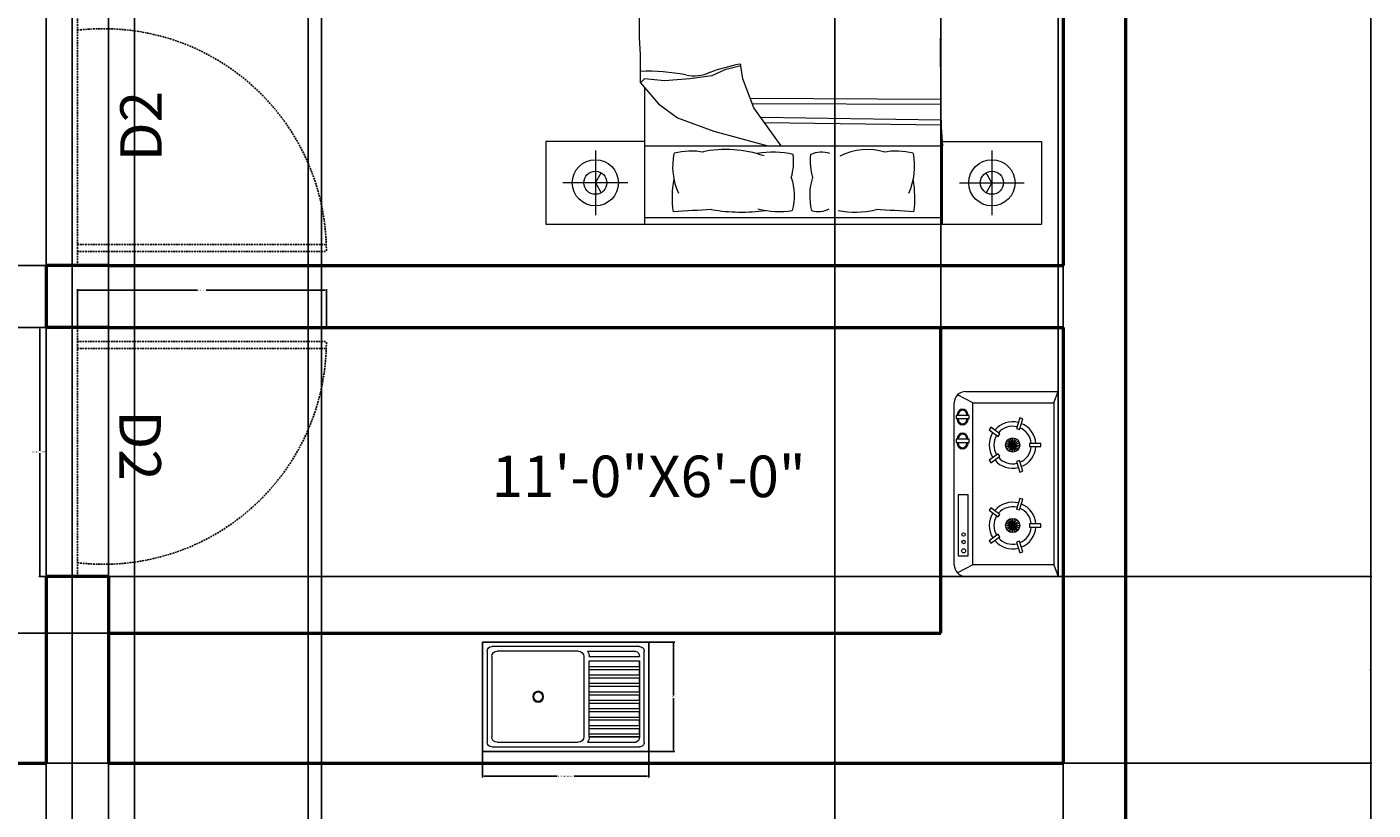
# Model space of a CAD drawing. Units: inches. Extents: x 3 to 576, y -689 to 51.
# Tile 19 of 21: x 381 to 576, y -261 to -148. Entities that reach past the tile are written whole.
import ezdxf

# ---------------------------------------------------------------- set-up
doc = ezdxf.new("R2010")
doc.units = ezdxf.units.IN
doc.header["$MEASUREMENT"] = 0
doc.linetypes.add('DASHED2', pattern=[0.375, 0.25, -0.125])
for name, color, linetype, lineweight in [('A-ANNO-DIMS', 2, 'Continuous', 18), ('A-ANNO-TEXT', 3, 'Continuous', 18), ('A-AREA-IDEN', 7, 'Continuous', 18), ('A-DOOR', 4, 'DASHED2', 25), ('A-EQPM', 8, 'Continuous', 18), ('A-FLOR-FIXT', 9, 'Continuous', 18), ('A-FURN', 8, 'Continuous', 18), ('A-WALL', 7, 'Continuous', 50)]:
    doc.layers.add(name, color=color, linetype=linetype, lineweight=lineweight)
doc.styles.get("Standard").update_dxf_attribs({"font": 'arial.ttf'})
doc.dimstyles.get("Standard").update_dxf_attribs({"dimtxt": 0.18, "dimasz": 0.18, "dimexe": 0.18, "dimexo": 0.0625, "dimgap": 0.09, "dimtad": 0, "dimtih": 1, "dimtoh": 1, "dimdec": 0, "dimzin": 0, "dimdsep": 46, "dimlunit": 3, "dimtxsty": 'Standard', "dimcen": 0.09, "dimadec": 0, "dimazin": 0, "dimtfac": 1, "dimtdec": 0, "dimtofl": 0, "dimtmove": 0, "dimatfit": 3, "dimfxl": 1, "dimtolj": 1, "dimtzin": 0, "dimarcsym": 0})

# ---------------------------------------------------------------- blocks, each defined once
blk = doc.blocks.new('М12 540х820')
for p, q in [((0, 540), (-820, 540)), ((-820, 540), (-820, 0)), ((0, 0), (0, 540)), ((-797.5, 495), (-797.5, 45)), ((-45, 517.5), (-775, 517.5)), ((-775, 468), (-775, 72)), ((-347.5, 495), (-748, 495)), ((-320.5, 468), (-320.5, 72)), ((-301.7, 495), (-64.8, 495)), ((-293.7, 468), (-293.7, 472.5)), ((-293.7, 468), (-45, 468)), ((-45, 469.5), (-45, 468)), ((-22.5, 45), (-22.5, 495)), ((-293.7, 446.6), (-45, 446.6)), ((-293.7, 419.6), (-293.7, 446.6)), ((-293.7, 419.6), (-45, 419.6)), ((-293.7, 405), (-45, 405)), ((-293.7, 378), (-293.7, 405)), ((-45, 419.6), (-45, 446.6)), ((-45, 378), (-45, 405)), ((-293.7, 378), (-45, 378)), ((-293.7, 336.4), (-293.7, 363.4)), ((-293.7, 363.4), (-45, 363.4)), ((-293.7, 336.4), (-45, 336.4)), ((-45, 336.4), (-45, 363.4)), ((-293.7, 294.7), (-293.7, 321.7)), ((-293.7, 321.7), (-45, 321.7)), ((-293.7, 294.7), (-45, 294.7)), ((-293.7, 253.1), (-293.7, 280.1)), ((-293.7, 280.1), (-45, 280.1)), ((-45, 294.7), (-45, 321.7)), ((-45, 253.1), (-45, 280.1)), ((-293.7, 253.1), (-45, 253.1)), ((-293.7, 211.5), (-293.7, 238.5)), ((-293.7, 238.5), (-45, 238.5)), ((-293.7, 211.5), (-45, 211.5)), ((-45, 211.5), (-45, 238.5)), ((-293.7, 169.9), (-293.7, 196.9)), ((-293.7, 196.9), (-45, 196.9)), ((-293.7, 169.9), (-45, 169.9)), ((-293.7, 128.2), (-293.7, 155.2)), ((-293.7, 155.2), (-45, 155.2)), ((-45, 169.9), (-45, 196.9)), ((-45, 128.2), (-45, 155.2)), ((-293.7, 128.2), (-45, 128.2)), ((-293.7, 113.6), (-45, 113.6)), ((-293.7, 86.6), (-293.7, 113.6)), ((-293.7, 86.6), (-45, 86.6)), ((-293.7, 72), (-45, 72)), ((-45, 86.6), (-45, 113.6)), ((-45, 70.5), (-45, 72)), ((-820, 0), (0, 0)), ((-775, 22.5), (-45, 22.5)), ((-748, 45), (-347.5, 45)), ((-301.7, 45), (-64.8, 45))]:
    blk.add_line(p, q)
at = {"ltscale": 0.06}
for p, q in [((-820, 0), (-820, 540)), ((-820, 540), (0, 540)), ((0, 540), (0, 536.9)), ((0, 536.9), (0, 0)), ((-293.7, 446.6), (-45, 446.6)), ((-293.7, 405), (-293.7, 446.6)), ((-293.7, 363.4), (-293.7, 405)), ((-45, 446.6), (-45, 419.6)), ((-45, 419.6), (-45, 378)), ((-293.7, 321.7), (-293.7, 363.4)), ((-45, 378), (-45, 336.4)), ((-45, 336.4), (-45, 294.7)), ((-293.7, 280.1), (-293.7, 321.7)), ((-293.7, 238.5), (-293.7, 280.1)), ((-45, 294.7), (-45, 253.1)), ((-293.7, 196.9), (-293.7, 238.5)), ((-45, 253.1), (-45, 211.5)), ((-45, 211.5), (-45, 169.9)), ((-293.7, 155.2), (-293.7, 196.9)), ((-293.7, 113.6), (-293.7, 155.2)), ((-45, 169.9), (-45, 128.2)), ((-293.7, 72), (-293.7, 113.6)), ((-45, 72), (-293.7, 72)), ((-45, 128.2), (-45, 86.6)), ((-45, 86.6), (-45, 72)), ((0, 0), (-820, 0))]:
    blk.add_line(p, q, dxfattribs=at)
at = {"extrusion": (0, 0, -1)}
for centre, major_axis, start_param, end_param in [((-775, 495), (-15.9, 15.9), -0.785398, 0.785398), ((-775, 495), (-15.9, 15.9), -0.785398, 0.785398), ((-748, 468), (-19.1, -19.1), 0.785398, 2.356194), ((-748, 468), (-19.1, -19.1), 0.785398, 2.356194), ((-347.5, 468), (-19.1, 19.1), 0.785398, 2.356194), ((-347.5, 468), (-19.1, 19.1), 0.785398, 2.356194), ((-343.2, 468), (-35, 35), 1.779263, 2.356194), ((-343.2, 468), (-35, 35), 1.779263, 2.356192), ((-343.2, 468), (-35, 35), 2.356192, 2.356194), ((-72.3, 468.8), (-19.3, 19.3), 1.0328, 2.38382), ((-72.3, 468.8), (-19.3, 19.3), 1.0328, 1.064673), ((-72.3, 468.8), (-19.3, 19.3), 1.064673, 2.328569), ((-45, 495), (-15.9, -15.9), 2.356194, 3.926991), ((-45, 495), (-15.9, -15.9), 2.356194, 3.926991), ((-72.3, 468.8), (-19.3, 19.3), 2.328569, 2.38382), ((-545.5, 270), (-19.1, -19.1), 3.926991, 10.210176), ((-545.5, 270), (-19.1, -19.1), 3.926991, 10.210176), ((-545.5, 270), (-15.9, -15.9), 3.926991, 10.210176), ((-545.5, 270), (-15.9, -15.9), 3.926991, 10.210176), ((-748, 72), (-19.1, 19.1), 3.926991, 5.497787), ((-748, 72), (-19.1, 19.1), 3.926991, 5.497787), ((-347.5, 72), (-19.1, -19.1), 3.926991, 5.497787), ((-347.5, 72), (-19.1, -19.1), 3.926991, 5.497787), ((-343.2, 72), (-35, -35), 3.926991, 4.503922), ((-343.2, 72), (-35, -35), 3.926991, 4.503922), ((-72.3, 71.2), (-19.3, -19.3), 3.899365, 5.250385), ((-72.3, 71.2), (-19.3, -19.3), 3.954617, 5.218512), ((-72.3, 71.2), (-19.3, -19.3), 3.899365, 3.954617), ((-775, 45), (-15.9, -15.9), 5.497787, 7.068583), ((-775, 45), (-15.9, -15.9), 5.497787, 7.068583), ((-72.3, 71.2), (-19.3, -19.3), 5.218512, 5.250385), ((-45, 45), (-15.9, 15.9), 2.356194, 3.926991), ((-45, 45), (-15.9, 15.9), 2.356194, 3.926991)]:
    blk.add_ellipse(centre, major_axis=major_axis, ratio=1, start_param=start_param, end_param=end_param, dxfattribs=at)
blk = doc.blocks.new('DOOR-SWING-900')
for p, q in [((35.95, 36), (35.95, 34)), ((36, 2), (35.95, 34)), ((36, 2), (0, 2)), ((36, 0), (36, 2))]:
    blk.add_line(p, q)
blk.add_arc((32.22, 2), 32.22, 83.347, 180)
blk = doc.blocks.new('*D15')
at = {"layer": 'A-ANNO-DIMS', "color": 0, "lineweight": -2, "transparency": 16777216}
for p, q in [((388.72, -191.31), (383.2, -191.31)), ((383.38, -191.49), (383.37, -209.12)), ((383.37, -227.13), (383.37, -209.49)), ((388.71, -227.31), (383.19, -227.31))]:
    blk.add_line(p, q, dxfattribs=at)
at = {"layer": 'A-ANNO-DIMS', "color": 0, "transparency": 16777216}
for points in [[(383.35, -191.49), (383.41, -191.49), (383.38, -191.31)], [(383.34, -227.13), (383.4, -227.13), (383.37, -227.31)]]:
    blk.add_solid(points, dxfattribs=at)
at = {"layer": 'Defpoints', "color": 0, "transparency": 16777216}
for p in [(388.78, -191.31), (383.37, -227.31), (388.77, -227.31)]:
    blk.add_point(p, dxfattribs=at)
at = {"layer": 'A-ANNO-DIMS', "color": 0, "transparency": 16777216, "insert": (383.37, -209.31), "char_height": 0.18, "attachment_point": 5}
blk.add_mtext('\\A1;DOOR D2 3\'-0" TYP.', dxfattribs=at)
blk = doc.blocks.new('*D16')
at = {"layer": 'A-ANNO-DIMS', "color": 0, "lineweight": -2, "transparency": 16777216}
for p, q in [((388.78, -191.25), (388.78, -185.73)), ((388.96, -185.91), (406.14, -185.91)), ((424.6, -185.92), (407.42, -185.91)), ((424.78, -191.25), (424.78, -185.74))]:
    blk.add_line(p, q, dxfattribs=at)
at = {"layer": 'A-ANNO-DIMS', "color": 0, "transparency": 16777216}
for points in [[(388.96, -185.88), (388.96, -185.94), (388.78, -185.91)], [(424.6, -185.89), (424.6, -185.95), (424.78, -185.92)]]:
    blk.add_solid(points, dxfattribs=at)
at = {"layer": 'Defpoints', "color": 0, "transparency": 16777216}
for p in [(388.78, -185.91), (388.78, -191.31), (424.78, -191.32)]:
    blk.add_point(p, dxfattribs=at)
at = {"layer": 'A-ANNO-DIMS', "color": 0, "transparency": 16777216, "insert": (406.78, -185.91), "char_height": 0.18, "attachment_point": 5}
blk.add_mtext('\\A1;3\'-0" TYP.', dxfattribs=at)
blk = doc.blocks.new('*D25')
at = {"layer": 'A-ANNO-DIMS', "color": 0, "lineweight": -2, "transparency": 16777216}
for p, q in [((447.36, -252.65), (447.36, -256.37)), ((471.37, -252.65), (471.37, -256.37)), ((447.54, -256.19), (458.13, -256.19)), ((471.19, -256.19), (460.61, -256.19))]:
    blk.add_line(p, q, dxfattribs=at)
at = {"layer": 'A-ANNO-DIMS', "color": 0, "transparency": 16777216}
for points in [[(447.54, -256.16), (447.54, -256.22), (447.36, -256.19)], [(471.19, -256.16), (471.19, -256.22), (471.37, -256.19)]]:
    blk.add_solid(points, dxfattribs=at)
at = {"layer": 'Defpoints', "color": 0, "transparency": 16777216}
for p in [(447.36, -252.59), (471.37, -252.59), (471.37, -256.19)]:
    blk.add_point(p, dxfattribs=at)
at = {"layer": 'A-ANNO-DIMS', "color": 0, "transparency": 16777216, "insert": (459.37, -256.19), "char_height": 0.18, "attachment_point": 5}
blk.add_mtext('\\A1;KITCHEN SINK 2\'-0"', dxfattribs=at)
blk = doc.blocks.new('*D26')
at = {"layer": 'A-ANNO-DIMS', "color": 0, "lineweight": -2, "transparency": 16777216}
for p, q in [((471.43, -236.78), (475.15, -236.78)), ((474.97, -236.96), (474.97, -244.5)), ((474.97, -252.41), (474.97, -244.87)), ((471.43, -252.59), (475.15, -252.59))]:
    blk.add_line(p, q, dxfattribs=at)
at = {"layer": 'A-ANNO-DIMS', "color": 0, "transparency": 16777216}
for points in [[(474.94, -236.96), (475, -236.96), (474.97, -236.78)], [(474.94, -252.41), (475, -252.41), (474.97, -252.59)]]:
    blk.add_solid(points, dxfattribs=at)
at = {"layer": 'Defpoints', "color": 0, "transparency": 16777216}
for p in [(471.37, -236.78), (474.97, -236.78), (471.37, -252.59)]:
    blk.add_point(p, dxfattribs=at)
at = {"layer": 'A-ANNO-DIMS', "color": 0, "transparency": 16777216, "insert": (474.97, -244.68), "char_height": 0.18, "attachment_point": 5}
blk.add_mtext('\\A1;1\'-4"', dxfattribs=at)
blk = doc.blocks.new('*D39')
at = {"layer": 'A-ANNO-DIMS', "color": 0, "lineweight": -2, "transparency": 16777216}
for p, q in [((540.36, 15.69), (575.92, 15.69)), ((575.74, 15.51), (575.74, -318.63)), ((575.74, -653.13), (575.74, -318.99)), ((540.36, -653.31), (575.92, -653.31))]:
    blk.add_line(p, q, dxfattribs=at)
at = {"layer": 'A-ANNO-DIMS', "color": 0, "transparency": 16777216}
for points in [[(575.71, 15.51), (575.77, 15.51), (575.74, 15.69)], [(575.71, -653.13), (575.77, -653.13), (575.74, -653.31)]]:
    blk.add_solid(points, dxfattribs=at)
at = {"layer": 'Defpoints', "color": 0, "transparency": 16777216}
for p in [(540.29, 15.69), (540.29, -653.31), (575.74, -653.31)]:
    blk.add_point(p, dxfattribs=at)
at = {"layer": 'A-ANNO-DIMS', "color": 0, "transparency": 16777216, "insert": (575.74, -318.81), "char_height": 0.18, "attachment_point": 5}
blk.add_mtext('\\A1;55\'-9"', dxfattribs=at)
blk = doc.blocks.new('*D65')
at = {"layer": 'A-ANNO-DIMS', "color": 0, "lineweight": -2, "transparency": 16777216}
for p, q in [((531.23, -50.31), (2.66, -50.31)), ((2.84, -50.49), (2.84, -116.13)), ((2.84, -182.13), (2.84, -116.49)), ((531.23, -182.31), (2.66, -182.31))]:
    blk.add_line(p, q, dxfattribs=at)
at = {"layer": 'A-ANNO-DIMS', "color": 0, "transparency": 16777216}
for points in [[(2.81, -50.49), (2.87, -50.49), (2.84, -50.31)], [(2.81, -182.13), (2.87, -182.13), (2.84, -182.31)]]:
    blk.add_solid(points, dxfattribs=at)
at = {"layer": 'Defpoints', "color": 0, "transparency": 16777216}
for p in [(531.29, -50.31), (2.84, -182.31), (531.29, -182.31)]:
    blk.add_point(p, dxfattribs=at)
at = {"layer": 'A-ANNO-DIMS', "color": 0, "transparency": 16777216, "insert": (2.84, -116.31), "char_height": 0.18, "attachment_point": 5}
blk.add_mtext('\\A1;11\'-0"', dxfattribs=at)
blk = doc.blocks.new('*D66')
at = {"layer": 'A-ANNO-DIMS', "color": 0, "lineweight": -2, "transparency": 16777216}
for p, q in [((531.23, -182.31), (2.66, -182.31)), ((2.84, -182.49), (2.84, -186.63)), ((2.84, -191.13), (2.84, -186.99)), ((531.23, -191.31), (2.66, -191.31))]:
    blk.add_line(p, q, dxfattribs=at)
at = {"layer": 'A-ANNO-DIMS', "color": 0, "transparency": 16777216}
for points in [[(2.81, -182.49), (2.87, -182.49), (2.84, -182.31)], [(2.81, -191.13), (2.87, -191.13), (2.84, -191.31)]]:
    blk.add_solid(points, dxfattribs=at)
at = {"layer": 'Defpoints', "color": 0, "transparency": 16777216}
for p in [(531.29, -182.31), (2.84, -191.31), (531.29, -191.31)]:
    blk.add_point(p, dxfattribs=at)
at = {"layer": 'A-ANNO-DIMS', "color": 0, "transparency": 16777216, "insert": (2.84, -186.81), "char_height": 0.18, "attachment_point": 5}
blk.add_mtext('\\A1;0\'-9"', dxfattribs=at)
blk = doc.blocks.new('*D67')
at = {"layer": 'A-ANNO-DIMS', "color": 0, "lineweight": -2, "transparency": 16777216}
for p, q in [((531.23, -191.31), (2.66, -191.31)), ((2.84, -191.49), (2.84, -222.63)), ((2.84, -254.13), (2.84, -222.99)), ((531.23, -254.31), (2.66, -254.31))]:
    blk.add_line(p, q, dxfattribs=at)
at = {"layer": 'A-ANNO-DIMS', "color": 0, "transparency": 16777216}
for points in [[(2.81, -191.49), (2.87, -191.49), (2.84, -191.31)], [(2.81, -254.13), (2.87, -254.13), (2.84, -254.31)]]:
    blk.add_solid(points, dxfattribs=at)
at = {"layer": 'Defpoints', "color": 0, "transparency": 16777216}
for p in [(531.29, -191.31), (2.84, -254.31), (531.29, -254.31)]:
    blk.add_point(p, dxfattribs=at)
at = {"layer": 'A-ANNO-DIMS', "color": 0, "transparency": 16777216, "insert": (2.84, -222.81), "char_height": 0.18, "attachment_point": 5}
blk.add_mtext('\\A1;5\'-3"', dxfattribs=at)
blk = doc.blocks.new('*D68')
at = {"layer": 'A-ANNO-DIMS', "color": 0, "lineweight": -2, "transparency": 16777216}
for p, q in [((531.23, -254.31), (2.66, -254.31)), ((2.84, -254.49), (2.84, -258.63)), ((2.84, -263.13), (2.84, -258.99)), ((531.23, -263.31), (2.66, -263.31))]:
    blk.add_line(p, q, dxfattribs=at)
at = {"layer": 'A-ANNO-DIMS', "color": 0, "transparency": 16777216}
for points in [[(2.81, -254.49), (2.87, -254.49), (2.84, -254.31)], [(2.81, -263.13), (2.87, -263.13), (2.84, -263.31)]]:
    blk.add_solid(points, dxfattribs=at)
at = {"layer": 'Defpoints', "color": 0, "transparency": 16777216}
for p in [(531.29, -254.31), (2.84, -263.31), (531.29, -263.31)]:
    blk.add_point(p, dxfattribs=at)
at = {"layer": 'A-ANNO-DIMS', "color": 0, "transparency": 16777216, "insert": (2.84, -258.81), "char_height": 0.18, "attachment_point": 5}
blk.add_mtext('\\A1;0\'-9"', dxfattribs=at)
blk = doc.blocks.new('*D94')
at = {"layer": 'A-ANNO-DIMS', "color": 0, "lineweight": -2, "transparency": 16777216}
for p, q in [((393.29, -136.9), (393.29, -688.94)), ((422.14, -136.9), (422.14, -688.94)), ((393.47, -688.76), (407.39, -688.76)), ((421.96, -688.76), (408.05, -688.76))]:
    blk.add_line(p, q, dxfattribs=at)
at = {"layer": 'A-ANNO-DIMS', "color": 0, "transparency": 16777216}
for points in [[(393.47, -688.73), (393.47, -688.79), (393.29, -688.76)], [(421.96, -688.73), (421.96, -688.79), (422.14, -688.76)]]:
    blk.add_solid(points, dxfattribs=at)
at = {"layer": 'Defpoints', "color": 0, "transparency": 16777216}
for p in [(393.29, -136.84), (422.14, -136.84), (422.14, -688.76)]:
    blk.add_point(p, dxfattribs=at)
at = {"layer": 'A-ANNO-DIMS', "color": 0, "transparency": 16777216, "insert": (407.72, -688.76), "char_height": 0.18, "attachment_point": 5}
blk.add_mtext('\\A1;2\'-5"', dxfattribs=at)
blk = doc.blocks.new('*D96')
at = {"layer": 'A-ANNO-DIMS', "color": 0, "lineweight": -2, "transparency": 16777216}
for p, q in [((397.02, -506.04), (397.02, 51.32)), ((397.2, 51.14), (410.22, 51.14)), ((423.91, 51.14), (410.89, 51.14)), ((424.09, -506.04), (424.09, 51.32))]:
    blk.add_line(p, q, dxfattribs=at)
at = {"layer": 'A-ANNO-DIMS', "color": 0, "transparency": 16777216}
for points in [[(397.2, 51.17), (397.2, 51.11), (397.02, 51.14)], [(423.91, 51.17), (423.91, 51.11), (424.09, 51.14)]]:
    blk.add_solid(points, dxfattribs=at)
at = {"layer": 'Defpoints', "color": 0, "transparency": 16777216}
for p in [(424.09, 51.14), (397.02, -506.1), (424.09, -506.1)]:
    blk.add_point(p, dxfattribs=at)
at = {"layer": 'A-ANNO-DIMS', "color": 0, "transparency": 16777216, "insert": (410.56, 51.14), "char_height": 0.18, "attachment_point": 5}
blk.add_mtext('\\A1;2\'-3"', dxfattribs=at)
blk = doc.blocks.new('*D103')
at = {"layer": 'A-ANNO-DIMS', "color": 0, "lineweight": -2, "transparency": 16777216}
for p, q in [((498.29, -50.37), (498.29, -688.94)), ((531.29, -50.37), (531.29, -688.94)), ((498.47, -688.76), (514.46, -688.76)), ((531.11, -688.76), (515.12, -688.76))]:
    blk.add_line(p, q, dxfattribs=at)
at = {"layer": 'A-ANNO-DIMS', "color": 0, "transparency": 16777216}
for points in [[(498.47, -688.73), (498.47, -688.79), (498.29, -688.76)], [(531.11, -688.73), (531.11, -688.79), (531.29, -688.76)]]:
    blk.add_solid(points, dxfattribs=at)
at = {"layer": 'Defpoints', "color": 0, "transparency": 16777216}
for p in [(498.29, -50.31), (531.29, -50.31), (531.29, -688.76)]:
    blk.add_point(p, dxfattribs=at)
at = {"layer": 'A-ANNO-DIMS', "color": 0, "transparency": 16777216, "insert": (514.79, -688.76), "char_height": 0.18, "attachment_point": 5}
blk.add_mtext('\\A1;2\'-9"', dxfattribs=at)
blk = doc.blocks.new('*D105')
at = {"layer": 'A-ANNO-DIMS', "color": 0, "lineweight": -2, "transparency": 16777216}
for p, q in [((393.36, -227.31), (575.92, -227.31)), ((575.74, -227.49), (575.74, -240.63)), ((575.74, -254.13), (575.74, -240.99)), ((393.36, -254.31), (575.92, -254.31))]:
    blk.add_line(p, q, dxfattribs=at)
at = {"layer": 'A-ANNO-DIMS', "color": 0, "transparency": 16777216}
for points in [[(575.71, -227.49), (575.77, -227.49), (575.74, -227.31)], [(575.71, -254.13), (575.77, -254.13), (575.74, -254.31)]]:
    blk.add_solid(points, dxfattribs=at)
at = {"layer": 'Defpoints', "color": 0, "transparency": 16777216}
for p in [(393.29, -227.31), (393.29, -254.31), (575.74, -254.31)]:
    blk.add_point(p, dxfattribs=at)
at = {"layer": 'A-ANNO-DIMS', "color": 0, "transparency": 16777216, "insert": (575.74, -240.81), "char_height": 0.18, "attachment_point": 5}
blk.add_mtext('\\A1;2\'-3"', dxfattribs=at)
blk = doc.blocks.new('*D116')
at = {"layer": 'A-ANNO-DIMS', "color": 0, "lineweight": -2, "transparency": 16777216}
for p, q in [((360.29, -134.37), (360.29, -688.94)), ((384.29, -134.37), (384.29, -688.94)), ((360.47, -688.76), (371.96, -688.76)), ((384.11, -688.76), (372.62, -688.76))]:
    blk.add_line(p, q, dxfattribs=at)
at = {"layer": 'A-ANNO-DIMS', "color": 0, "transparency": 16777216}
for points in [[(360.47, -688.73), (360.47, -688.79), (360.29, -688.76)], [(384.11, -688.73), (384.11, -688.79), (384.29, -688.76)]]:
    blk.add_solid(points, dxfattribs=at)
at = {"layer": 'Defpoints', "color": 0, "transparency": 16777216}
for p in [(360.29, -134.31), (384.29, -134.31), (384.29, -688.76)]:
    blk.add_point(p, dxfattribs=at)
at = {"layer": 'A-ANNO-DIMS', "color": 0, "transparency": 16777216, "insert": (372.29, -688.76), "char_height": 0.18, "attachment_point": 5}
blk.add_mtext('\\A1;2\'-0"', dxfattribs=at)
blk = doc.blocks.new('*D118')
at = {"layer": 'A-ANNO-DIMS', "color": 0, "lineweight": -2, "transparency": 16777216}
for p, q in [((352.02, -506.25), (352.02, 51.32)), ((352.2, 51.14), (369.69, 51.14)), ((387.84, 51.14), (370.35, 51.14)), ((388.02, -506.25), (388.02, 51.32))]:
    blk.add_line(p, q, dxfattribs=at)
at = {"layer": 'A-ANNO-DIMS', "color": 0, "transparency": 16777216}
for points in [[(352.2, 51.17), (352.2, 51.11), (352.02, 51.14)], [(387.84, 51.17), (387.84, 51.11), (388.02, 51.14)]]:
    blk.add_solid(points, dxfattribs=at)
at = {"layer": 'Defpoints', "color": 0, "transparency": 16777216}
for p in [(388.02, 51.14), (352.02, -506.31), (388.02, -506.31)]:
    blk.add_point(p, dxfattribs=at)
at = {"layer": 'A-ANNO-DIMS', "color": 0, "transparency": 16777216, "insert": (370.02, 51.14), "char_height": 0.18, "attachment_point": 5}
blk.add_mtext('\\A1;3\'-0"', dxfattribs=at)
blk = doc.blocks.new('*D123')
at = {"layer": 'A-ANNO-DIMS', "color": 0, "lineweight": -2, "transparency": 16777216}
for p, q in [((513.55, -235.5), (2.66, -235.5)), ((2.84, -235.68), (2.84, -244.72)), ((2.84, -254.13), (2.84, -245.08)), ((531.23, -254.31), (2.66, -254.31))]:
    blk.add_line(p, q, dxfattribs=at)
at = {"layer": 'A-ANNO-DIMS', "color": 0, "transparency": 16777216}
for points in [[(2.81, -235.68), (2.87, -235.68), (2.84, -235.5)], [(2.81, -254.13), (2.87, -254.13), (2.84, -254.31)]]:
    blk.add_solid(points, dxfattribs=at)
at = {"layer": 'Defpoints', "color": 0, "transparency": 16777216}
for p in [(513.61, -235.5), (2.84, -254.31), (531.29, -254.31)]:
    blk.add_point(p, dxfattribs=at)
at = {"layer": 'A-ANNO-DIMS', "color": 0, "transparency": 16777216, "insert": (2.84, -244.9), "char_height": 0.18, "attachment_point": 5}
blk.add_mtext('\\A1;1\'-7"', dxfattribs=at)
blk = doc.blocks.new('*D124')
at = {"layer": 'A-ANNO-DIMS', "color": 0, "lineweight": -2, "transparency": 16777216}
for p, q in [((513.61, -235.44), (513.61, 51.32)), ((513.79, 51.14), (521.77, 51.14)), ((530.39, 51.14), (522.41, 51.14)), ((530.57, -227.22), (530.57, 51.32))]:
    blk.add_line(p, q, dxfattribs=at)
at = {"layer": 'A-ANNO-DIMS', "color": 0, "transparency": 16777216}
for points in [[(513.79, 51.17), (513.79, 51.11), (513.61, 51.14)], [(530.39, 51.17), (530.39, 51.11), (530.57, 51.14)]]:
    blk.add_solid(points, dxfattribs=at)
at = {"layer": 'Defpoints', "color": 0, "transparency": 16777216}
for p in [(530.57, 51.14), (530.57, -227.28), (513.61, -235.5)]:
    blk.add_point(p, dxfattribs=at)
at = {"layer": 'A-ANNO-DIMS', "color": 0, "transparency": 16777216, "insert": (522.09, 51.14), "char_height": 0.18, "attachment_point": 5}
blk.add_mtext('\\A1;1\'-5"', dxfattribs=at)

msp = doc.modelspace()

# ---------------------------------------------------------------- linework, layer by layer
at = {"layer": 'A-DOOR'}
for p, q in [((388.79, -179.31), (424.79, -179.31)), ((388.79, -194.31), (424.79, -194.31))]:
    msp.add_line(p, q, dxfattribs=at)
at = {"layer": 'A-EQPM'}
for p, q in [((515.53, -225.61), (515.53, -202.21)), ((518.23, -202.21), (516.01, -201.03)), ((517.2, -200.54), (530.57, -200.54)), ((518.23, -202.21), (529.93, -202.21)), ((518.23, -225.61), (518.23, -202.21)), ((529.93, -202.21), (530.57, -200.54)), ((529.93, -202.21), (529.93, -225.61)), ((530.57, -200.54), (530.57, -227.28)), ((517.68, -204), (515.83, -204)), ((515.83, -204), (515.83, -204.43)), ((517.68, -204.43), (517.68, -204)), ((515.83, -204.43), (517.68, -204.43)), ((520.83, -205.72), (520.57, -206.09)), ((520.57, -206.09), (521.88, -207.04)), ((522.15, -206.67), (520.83, -205.72)), ((525.02, -204.36), (524.52, -205.9)), ((524.52, -205.9), (524.95, -206.04)), ((524.95, -206.04), (525.46, -204.5)), ((525.46, -204.5), (525.02, -204.36)), ((517.68, -207.46), (515.83, -207.46)), ((515.83, -207.46), (515.83, -207.9)), ((515.83, -207.9), (517.68, -207.9)), ((517.68, -207.9), (517.68, -207.46)), ((521.88, -207.04), (522.15, -206.67)), ((523.98, -208.29), (523.01, -207.97)), ((523.98, -208.29), (523.15, -207.68)), ((523.98, -208.29), (523.38, -207.46)), ((523.98, -208.29), (523.67, -207.31)), ((523.98, -208.29), (523.98, -207.26)), ((523.98, -208.29), (524.3, -207.31)), ((523.98, -208.29), (524.59, -207.46)), ((523.98, -208.29), (524.82, -207.68)), ((523.98, -208.29), (524.96, -207.97)), ((526.42, -208.06), (526.42, -208.52)), ((528.04, -208.06), (526.42, -208.06)), ((528.04, -208.52), (528.04, -208.06)), ((521.88, -209.54), (520.57, -210.49)), ((520.83, -210.86), (522.15, -209.91)), ((522.15, -209.91), (521.88, -209.54)), ((523.98, -208.29), (522.96, -208.29)), ((523.98, -208.29), (523.01, -208.61)), ((523.98, -208.29), (523.15, -208.89)), ((523.98, -208.29), (523.38, -209.12)), ((523.98, -208.29), (523.67, -209.27)), ((523.98, -208.29), (523.98, -209.32)), ((523.98, -208.29), (524.3, -209.27)), ((523.98, -208.29), (524.59, -209.12)), ((523.98, -208.29), (524.82, -208.89)), ((523.98, -208.29), (524.96, -208.61)), ((523.98, -208.29), (525.01, -208.29)), ((526.42, -208.52), (528.04, -208.52)), ((520.57, -210.49), (520.83, -210.86)), ((524.95, -210.54), (524.52, -210.68)), ((524.52, -210.68), (525.02, -212.22)), ((525.46, -212.08), (524.95, -210.54)), ((525.02, -212.22), (525.46, -212.08)), ((516.1, -215.48), (516.1, -224.33)), ((517.53, -215.48), (516.1, -215.48)), ((517.53, -224.33), (517.53, -215.48)), ((520.83, -217.36), (520.57, -217.73)), ((520.57, -217.73), (521.88, -218.68)), ((522.15, -218.31), (520.83, -217.36)), ((525.02, -216), (524.52, -217.54)), ((524.52, -217.54), (524.95, -217.68)), ((524.95, -217.68), (525.46, -216.14)), ((525.46, -216.14), (525.02, -216)), ((521.88, -218.68), (522.15, -218.31)), ((523.98, -219.93), (523.01, -219.61)), ((523.98, -219.93), (523.15, -219.33)), ((523.98, -219.93), (523.38, -219.1)), ((523.98, -219.93), (523.67, -218.95)), ((523.98, -219.93), (523.98, -218.9)), ((523.98, -219.93), (524.3, -218.95)), ((523.98, -219.93), (524.59, -219.1)), ((523.98, -219.93), (524.82, -219.33)), ((523.98, -219.93), (524.96, -219.61)), ((526.42, -219.7), (526.42, -220.16)), ((528.04, -219.7), (526.42, -219.7)), ((528.04, -220.16), (528.04, -219.7)), ((521.88, -221.18), (520.57, -222.13)), ((520.83, -222.5), (522.15, -221.55)), ((522.15, -221.55), (521.88, -221.18)), ((523.98, -219.93), (522.96, -219.93)), ((523.98, -219.93), (523.01, -220.25)), ((523.98, -219.93), (523.15, -220.54)), ((523.98, -219.93), (523.38, -220.76)), ((523.98, -219.93), (523.67, -220.91)), ((523.98, -219.93), (525.01, -219.93)), ((523.98, -219.93), (524.96, -220.25)), ((523.98, -219.93), (524.82, -220.54)), ((523.98, -219.93), (524.59, -220.76)), ((523.98, -219.93), (524.3, -220.91)), ((523.98, -219.93), (523.98, -220.96)), ((526.42, -220.16), (528.04, -220.16)), ((520.57, -222.13), (520.83, -222.5)), ((524.95, -222.18), (524.52, -222.32)), ((524.52, -222.32), (525.02, -223.86)), ((525.46, -223.72), (524.95, -222.18)), ((525.02, -223.86), (525.46, -223.72)), ((518.23, -225.61), (516.01, -226.79)), ((516.1, -224.33), (517.53, -224.33)), ((529.93, -225.61), (518.23, -225.61)), ((529.93, -225.61), (530.57, -227.28)), ((530.57, -227.28), (517.2, -227.28))]:
    msp.add_line(p, q, dxfattribs=at)
for centre, radius in [((523.98, -208.29), 1.03), ((523.98, -219.93), 1.03), ((516.89, -221.22), 0.247), ((516.89, -223.59), 0.296), ((516.89, -222.31), 0.247)]:
    msp.add_circle(centre, radius, dxfattribs=at)
for centre, radius, start, end in [((517.2, -202.21), 1.67, 90, 180), ((523.98, -208.29), 3.37, 75.8765, 140.1235), ((523.98, -208.29), 2.71, 76.8365, 139.1635), ((523.98, -208.29), 2.71, 4.8365, 67.1635), ((523.98, -208.29), 3.37, 3.8765, 68.1235), ((523.98, -208.29), 3.37, 147.8765, 212.1235), ((523.98, -208.29), 2.71, 148.8365, 211.1635), ((523.98, -208.29), 2.71, 220.8365, 283.1635), ((523.98, -208.29), 2.71, 292.8365, 355.1635), ((523.98, -208.29), 3.37, 291.8765, 356.1235), ((523.98, -208.29), 3.37, 219.8765, 284.1235), ((523.98, -219.93), 3.37, 75.8765, 140.1235), ((523.98, -219.93), 2.71, 76.8365, 139.1635), ((523.98, -219.93), 2.71, 4.8365, 67.1635), ((523.98, -219.93), 3.37, 3.8765, 68.1235), ((523.98, -219.93), 3.37, 147.8765, 212.1235), ((523.98, -219.93), 2.71, 148.8365, 211.1635), ((523.98, -219.93), 2.71, 220.8365, 283.1635), ((523.98, -219.93), 2.71, 292.8365, 355.1635), ((523.98, -219.93), 3.37, 291.8765, 356.1235), ((523.98, -219.93), 3.37, 219.8765, 284.1235), ((517.2, -225.61), 1.67, 180, 270)]:
    msp.add_arc(centre, radius, start, end, dxfattribs=at)
at = {"layer": 'A-EQPM', "extrusion": (0, 0, -1)}
for centre, major_axis, start_param, end_param in [((516.74, -204.24), (0, -1.2), 1.774361, 4.508825), ((516.74, -204.24), (0, 1.2), 1.73081, 4.552375), ((516.74, -207.71), (0, 1.2), 1.73081, 4.552375), ((516.74, -207.71), (0, -1.2), 1.774361, 4.508825)]:
    msp.add_ellipse(centre, major_axis=major_axis, ratio=0.671641, start_param=start_param, end_param=end_param, dxfattribs=at)
at = {"layer": 'A-EQPM'}
for points, knots in [([(516.12, -204), (516.13, -203.94), (516.15, -203.89), (516.18, -203.76), (516.21, -203.69), (516.26, -203.57), (516.3, -203.51), (516.37, -203.41), (516.41, -203.37), (516.49, -203.3), (516.53, -203.27), (516.61, -203.23), (516.65, -203.22), (516.73, -203.21), (516.77, -203.21), (516.85, -203.23), (516.9, -203.24), (516.98, -203.29), (517.02, -203.32), (517.1, -203.39), (517.14, -203.44), (517.21, -203.54), (517.24, -203.6), (517.29, -203.73), (517.32, -203.8), (517.35, -203.91), (517.35, -203.96), (517.36, -204)], [8.079302, 8.079302, 8.079302, 8.079302, 8.245651, 8.245651, 8.463703, 8.463703, 8.681755, 8.681755, 8.899807, 8.899807, 9.117859, 9.117859, 9.33591, 9.33591, 9.553962, 9.553962, 9.772014, 9.772014, 9.990066, 9.990066, 10.208118, 10.208118, 10.426169, 10.426169, 10.644221, 10.644221, 10.770253, 10.770253, 10.770253, 10.770253]), ([(517.37, -204.43), (517.36, -204.48), (517.35, -204.52), (517.33, -204.64), (517.31, -204.71), (517.26, -204.84), (517.23, -204.91), (517.16, -205.02), (517.12, -205.06), (517.05, -205.15), (517, -205.18), (516.92, -205.23), (516.88, -205.25), (516.81, -205.27), (516.78, -205.27), (516.74, -205.27), (516.7, -205.27), (516.66, -205.27), (516.58, -205.24), (516.54, -205.22), (516.46, -205.16), (516.42, -205.13), (516.34, -205.04), (516.3, -204.99), (516.24, -204.87), (516.21, -204.81), (516.16, -204.67), (516.14, -204.6), (516.13, -204.49), (516.12, -204.46), (516.12, -204.43)], [4.889299, 4.889299, 4.889299, 4.889299, 5.015191, 5.015191, 5.233243, 5.233243, 5.451295, 5.451295, 5.669347, 5.669347, 5.887399, 5.887399, 6.10545, 6.10545, 6.283185, 6.283185, 6.283185, 6.501237, 6.501237, 6.719289, 6.719289, 6.937341, 6.937341, 7.155392, 7.155392, 7.373444, 7.373444, 7.591496, 7.591496, 7.677072, 7.677072, 7.677072, 7.677072]), ([(516.12, -207.46), (516.13, -207.41), (516.15, -207.35), (516.18, -207.22), (516.21, -207.15), (516.26, -207.03), (516.3, -206.97), (516.37, -206.87), (516.41, -206.83), (516.49, -206.76), (516.53, -206.74), (516.61, -206.7), (516.65, -206.68), (516.73, -206.67), (516.77, -206.68), (516.85, -206.69), (516.9, -206.71), (516.98, -206.75), (517.02, -206.78), (517.1, -206.85), (517.14, -206.9), (517.21, -207), (517.24, -207.06), (517.29, -207.19), (517.32, -207.26), (517.35, -207.38), (517.35, -207.42), (517.36, -207.46)], [8.079302, 8.079302, 8.079302, 8.079302, 8.245651, 8.245651, 8.463703, 8.463703, 8.681755, 8.681755, 8.899807, 8.899807, 9.117859, 9.117859, 9.33591, 9.33591, 9.553962, 9.553962, 9.772014, 9.772014, 9.990066, 9.990066, 10.208118, 10.208118, 10.426169, 10.426169, 10.644221, 10.644221, 10.770253, 10.770253, 10.770253, 10.770253]), ([(517.37, -207.9), (517.36, -207.94), (517.35, -207.98), (517.33, -208.1), (517.31, -208.17), (517.26, -208.31), (517.23, -208.37), (517.16, -208.48), (517.12, -208.53), (517.05, -208.61), (517, -208.64), (516.92, -208.69), (516.88, -208.71), (516.81, -208.73), (516.78, -208.73), (516.74, -208.73), (516.7, -208.73), (516.66, -208.73), (516.58, -208.7), (516.54, -208.68), (516.46, -208.62), (516.42, -208.59), (516.34, -208.5), (516.3, -208.45), (516.24, -208.34), (516.21, -208.27), (516.16, -208.13), (516.14, -208.06), (516.13, -207.96), (516.12, -207.93), (516.12, -207.9)], [4.889299, 4.889299, 4.889299, 4.889299, 5.015191, 5.015191, 5.233243, 5.233243, 5.451295, 5.451295, 5.669347, 5.669347, 5.887399, 5.887399, 6.10545, 6.10545, 6.283185, 6.283185, 6.283185, 6.501237, 6.501237, 6.719289, 6.719289, 6.937341, 6.937341, 7.155392, 7.155392, 7.373444, 7.373444, 7.591496, 7.591496, 7.677072, 7.677072, 7.677072, 7.677072])]:
    msp.add_open_spline(points, degree=3, knots=knots, dxfattribs=at)
at = {"layer": 'A-FURN'}
for p, q in [((484.7, -153.46), (482.38, -154.04)), ((484.99, -155.34), (484.7, -153.46)), ((470.76, -155.34), (470.18, -155.92)), ((473.67, -155.63), (470.76, -155.34)), ((477.3, -155.34), (473.67, -155.63)), ((480.49, -154.91), (477.3, -155.34)), ((482.38, -154.04), (480.49, -154.91)), ((486.59, -159.55), (484.99, -155.34)), ((470.18, -155.92), (472.8, -158.97)), ((470.83, -176.34), (470.83, -156.67)), ((472.8, -158.97), (475.55, -161)), ((513.57, -158.31), (486.07, -158.2)), ((513.57, -159.05), (486.35, -158.94)), ((490.51, -165.02), (486.59, -159.55)), ((475.55, -161), (480.78, -162.89)), ((513.61, -161.3), (487.58, -160.94)), ((480.78, -162.89), (488.6, -165.02)), ((513.63, -162.04), (488.12, -161.68)), ((470.83, -165.02), (513.83, -165.02)), ((463.66, -165.69), (463.66, -175.05)), ((520.99, -165.69), (520.99, -175.05)), ((468.34, -170.37), (458.98, -170.37)), ((516.31, -170.37), (525.67, -170.37)), ((456.49, -176.34), (528.16, -176.34)), ((513.83, -175.42), (470.83, -175.42))]:
    msp.add_line(p, q, dxfattribs=at)
for points in [[(470.03, -149.36, -0.001242), (470, -135.76, 0.127202), (468.56, -128.99)], [(474.94, -174.56, -0.074897), (475.03, -169.87, 0.472817)], [(491.99, -169.61, -0.14099), (492.13, -174.39, -0.235245)], [(495.05, -169.61, 0.14099), (494.91, -174.39, 0.235245)], [(509.71, -174.56, 0.074897), (509.62, -169.87, -0.472817)]]:
    msp.add_lwpolyline(points, format="xyb", dxfattribs=at)
for points in [[(470.83, -164.4), (456.49, -164.4), (456.49, -176.34)], [(513.83, -176.34), (513.83, -164.4), (528.16, -164.4), (528.16, -176.34)], [(463.66, -170.37), (464.49, -168.92)], [(520.99, -170.37), (520.16, -168.92)], [(463.66, -170.37), (464.49, -171.82)], [(520.99, -170.37), (520.16, -171.82)]]:
    msp.add_lwpolyline(points, dxfattribs=at)
for centre, radius in [((463.66, -170.37), 3.34), ((520.99, -170.37), 3.34), ((463.66, -170.37), 1.67), ((520.99, -170.37), 1.67)]:
    msp.add_circle(centre, radius, dxfattribs=at)
for centre, radius, start, end in [((681.5, -151.58), 167.98, 175.1265, 180.8855), ((404.47, -154.14), 65.74, 358.447, 4.1706), ((489.68, -180.54), 27.79, 100.6617, 109.8806), ((484.54, -153.4), 0.173, 340.2464, 91.1377), ((471.41, -181.3), 27.05, 78.6608, 92.5481), ((477.88, -149.06), 5.83, 258.6608, 293.7384), ((642.3, -156.26), 128.77, 179.0718, 183.9), ((484.07, -168), 9.24, 168.2417, 204.8684), ((477.5, -175.39), 9.6, 78.9631, 104.8961), ((482.55, -182.22), 16.66, 70.7385, 101.9603), ((489.3, -178.58), 12.64, 76.3762, 100.1383), ((483.54, -167.22), 8.78, 344.1707, 5.9871), ((503.5, -167.22), 8.78, 174.0129, 195.8293), ((496.37, -169.75), 3.8, 71.4593, 114.9817), ((503.01, -174.69), 9.12, 73.8254, 116.1239), ((507.15, -175.39), 9.6, 75.1039, 101.0369), ((500.58, -168), 9.24, 335.1316, 11.7583), ((514.44, -856.59), 683.18, 92.85022, 93.31479), ((484.76, -148.62), 25.99, 260.503, 277.7804), ((490.25, -161.76), 12.77, 256.04, 278.4751), ((495.89, -170.98), 3.55, 253.8974, 296.6563), ((501.2, -162.02), 12.6, 258.8159, 283.6573), ((470.21, -856.59), 683.18, 86.68521, 87.14978)]:
    msp.add_arc(centre, radius, start, end, dxfattribs=at)
at = {"layer": 'A-WALL'}
for p, q in [((540.29, 15.69), (540.29, -653.31)), ((531.29, -50.31), (531.29, -182.31)), ((393.29, -182.31), (384.29, -182.31)), ((384.29, -182.31), (384.29, -191.31)), ((393.29, -182.31), (465.29, -182.31)), ((465.29, -182.31), (474.29, -182.31)), ((474.29, -182.31), (531.29, -182.31)), ((393.29, -191.31), (384.29, -191.31)), ((393.29, -191.31), (465.29, -191.31)), ((465.29, -191.31), (474.29, -191.31)), ((474.29, -191.31), (531.29, -191.31)), ((513.61, -235.5), (513.61, -191.31)), ((531.29, -191.31), (531.29, -254.31)), ((393.29, -227.31), (384.29, -227.31)), ((384.29, -227.31), (384.29, -254.31)), ((393.29, -227.31), (393.29, -254.31)), ((393.29, -235.5), (513.61, -235.5)), ((372.29, -254.31), (384.29, -254.31)), ((393.29, -254.31), (531.29, -254.31))]:
    msp.add_line(p, q, dxfattribs=at)

# ---------------------------------------------------------------- block references
at = {"layer": 'A-DOOR', "extrusion": (0, 0, -1), "zscale": -1, "rotation": 359.9872034024854}
msp.add_blockref('DOOR-SWING-900', (-424.78, -182.3), dxfattribs=at)
at = {"layer": 'A-DOOR', "rotation": 179.9872034024853}
msp.add_blockref('DOOR-SWING-900', (424.78, -191.32), dxfattribs=at)
at = {"layer": 'A-FLOR-FIXT', "xscale": 0.0292793774279423, "yscale": 0.0292793774279423, "zscale": 0.0292793774279423}
msp.add_blockref('М12 540х820', (471.37, -252.59), dxfattribs=at)

# ---------------------------------------------------------------- texts
at = {"layer": 'A-ANNO-TEXT', "char_height": 6, "attachment_point": 1}
for insert, rotation in [((394.98, -167.27), 90), ((400.86, -203.27), 270)]:
    msp.add_mtext('D2', dxfattribs=dict(at, insert=insert, rotation=rotation))
at = {"layer": 'A-AREA-IDEN', "insert": (448.67, -209.82), "char_height": 6, "attachment_point": 1}
msp.add_mtext('11\'-0"X6\'-0"', dxfattribs=at)

# ---------------------------------------------------------------- dimensions: what is measured, and where the dimension line sits
at = {"layer": 'A-ANNO-DIMS'}
for base, p1, p2, picture, middle in [((388.02, 51.14), (352.02, -506.31), (388.02, -506.31), '*D118', (370.02, 51.14)), ((424.09, 51.14), (397.02, -506.1), (424.09, -506.1), '*D96', (410.56, 51.14)), ((530.57, 51.14), (513.61, -235.5), (530.57, -227.28), '*D124', (522.09, 51.14)), ((531.29, -688.76), (498.29, -50.31), (531.29, -50.31), '*D103', (514.79, -688.76)), ((384.29, -688.76), (360.29, -134.31), (384.29, -134.31), '*D116', (372.29, -688.76)), ((422.1383, -688.7597), (393.294, -136.8425), (422.1383, -136.8425), '*D94', (407.7162, -688.7597))]:
    dim = msp.add_linear_dim(base=base, p1=p1, p2=p2, dimstyle='Standard', override={"dimdec": 1, "dimlfac": 1, "dimrnd": 0, "dimzin": 1, "dimdsep": 46, "dimlunit": 4, "dimfrac": 2}, dxfattribs=at)
    dim.commit()
    dim.dimension.update_dxf_attribs({"geometry": picture, "text_midpoint": middle})
for base, p1, p2, picture, middle in [((575.74, -653.31), (540.29, 15.69), (540.29, -653.31), '*D39', (575.74, -318.81)), ((2.84, -182.31), (531.29, -50.31), (531.29, -182.31), '*D65', (2.84, -116.31)), ((2.84, -191.31), (531.29, -182.31), (531.29, -191.31), '*D66', (2.84, -186.81)), ((2.84, -254.31), (531.29, -191.31), (531.29, -254.31), '*D67', (2.84, -222.81)), ((575.74, -254.31), (393.29, -227.31), (393.29, -254.31), '*D105', (575.74, -240.81)), ((2.84, -254.31), (513.61, -235.5), (531.29, -254.31), '*D123', (2.84, -244.9)), ((474.97, -236.78), (471.37, -252.59), (471.37, -236.78), '*D26', (474.97, -244.68)), ((2.84, -263.31), (531.29, -254.31), (531.29, -263.31), '*D68', (2.84, -258.81))]:
    dim = msp.add_linear_dim(base=base, p1=p1, p2=p2, angle=90, dimstyle='Standard', override={"dimdec": 1, "dimlfac": 1, "dimrnd": 0, "dimzin": 1, "dimdsep": 46, "dimlunit": 4, "dimfrac": 2}, dxfattribs=at)
    dim.commit()
    dim.dimension.update_dxf_attribs({"geometry": picture, "text_midpoint": middle})
for base, p1, p2, angle, text, picture, middle in [((388.78, -185.91), (424.78, -191.32), (388.78, -191.31), 179.9872, '<> TYP.', '*D16', (406.78, -185.91)), ((383.37, -227.31), (388.78, -191.31), (388.77, -227.31), 269.9872, 'DOOR D2 <> TYP.', '*D15', (383.37, -209.31))]:
    dim = msp.add_linear_dim(base=base, p1=p1, p2=p2, angle=angle, text=text, dimstyle='Standard', override={"dimdec": 1, "dimlfac": 1, "dimrnd": 0, "dimzin": 1, "dimdsep": 46, "dimlunit": 4, "dimfrac": 2}, dxfattribs=at)
    dim.commit()
    dim.dimension.update_dxf_attribs({"geometry": picture, "text_midpoint": middle})
dim = msp.add_linear_dim(base=(471.37, -256.19), p1=(447.36, -252.59), p2=(471.37, -252.59), text='KITCHEN SINK <>', dimstyle='Standard', override={"dimdec": 1, "dimlfac": 1, "dimrnd": 0, "dimzin": 1, "dimdsep": 46, "dimlunit": 4, "dimfrac": 2}, dxfattribs=at)
dim.commit()
dim.dimension.update_dxf_attribs({"geometry": '*D25', "text_midpoint": (459.37, -256.19)})

doc.saveas('drawing.dxf')
